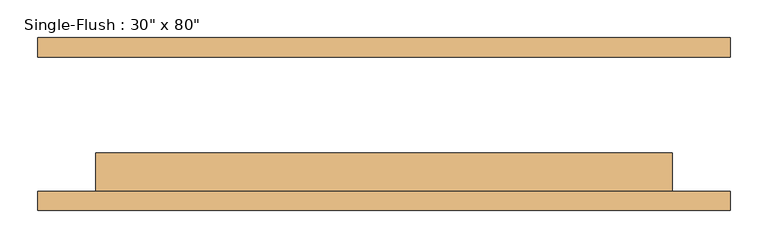
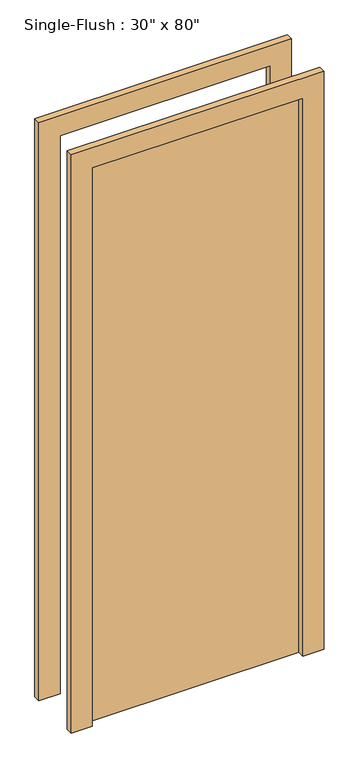
"""IFC4 building model written with IfcOpenShell, lengths in millimetres: door geometry."""

from ifc_helpers import new_model, si_unit, frame, origin, origin_with_axes, place, context, project, spatial, polyline, outline, extrude, source, transform, mapped, element, save


def door_b1104dde(model_context):
    return source(origin(), model_context, "Body", "SweptSolid", [
        extrude(outline(polyline([(2209.8, -457.2), (0.0, -457.2), (0.0, -381.0), (2133.6, -381.0), (2133.6, 381.0), (0.0, 381.0), (0.0, 457.2), (2209.8, 457.2), (2209.8, -457.2)])), frame((0.0, -114.3, 0.0), z_axis=(0.0, 1.0, 0.0), x_axis=(0.0, 0.0, 1.0)), (0.0, 0.0, 1.0), 25.4),
        extrude(outline(polyline([(2209.8, 457.2), (2209.8, -457.2), (0.0, -457.2), (0.0, -381.0), (2133.6, -381.0), (2133.6, 381.0), (0.0, 381.0), (0.0, 457.2), (2209.8, 457.2)])), frame((0.0, 88.9, 0.0), z_axis=(0.0, 1.0, 0.0), x_axis=(0.0, 0.0, 1.0)), (0.0, 0.0, 1.0), 25.4),
        extrude(outline(polyline([(381.0, -38.1), (381.0, -88.9), (-381.0, -88.9), (-381.0, -38.1), (381.0, -38.1)])), origin_with_axes(), (0.0, 0.0, 1.0), 2133.6),
    ])


if __name__ == "__main__":
    model = new_model("IFC4")
    model_context = context("Model", 3, world=origin())
    ifc_project = project(units=[si_unit("LENGTHUNIT", "METRE", prefix="MILLI")], contexts=[model_context])
    site = spatial("IfcSite", under=ifc_project)
    building = spatial("IfcBuilding", under=site)
    placement = place(None, origin())
    door_shape = door_b1104dde(model_context)
    element("IfcDoor", 1, ObjectType="Single-Flush : 30\" x 80\"", at=placement, inside=building, context=model_context, shape_type="MappedRepresentation", body=[
        mapped(door_shape, transform((0.0, 0.0, 0.0), x_axis=(1.0, 0.0, 0.0), y_axis=(0.0, 1.0, 0.0), z_axis=(0.0, 0.0, 1.0))),
    ])
    save(model, "model.ifc")

# Revit data of these elements
# Type "Single-Flush : 30\" x 80\""
#   Type Mark = "5"
#   Construction Type Id = "MDOOR"
#   Assembly Code = "C1020"
#   Analytic Construction = "Metal"
#   Thickness = 0' - 2"
#   Heat Transfer Coefficient (U) = 0.651978 BTU/(h·ft²·°F)
#   Height = 7' - 0"
#   Trim Projection Ext = 0' - 1"
#   Trim Projection Int = 0' - 1"
#   Trim Width = 0' - 3"
#   Width = 2' - 6"
#   Define Thermal Properties by = 1
#   Define Thermal Properties by = 1
#   Door Material = Door - Panel
#   Frame Material = Door - Frame
#   Visual Light Transmittance = 0
#   Solar Heat Gain Coefficient = 0
#   Function = (empty or 0)
#   Wall Closure = (empty or 0)
# Element 1 (IfcDoor, "Single-Flush : 30\" x 80\"")
#   Materials on its faces: "Door - Frame", "Door - Panel"
# Materials
#   "Door - Panel": class "Wood", colour RGB 210 159 95, transparency 0, Cost = 0
#   "Door - Frame": colour RGB 118 70 51, transparency 0, Cost = 0
